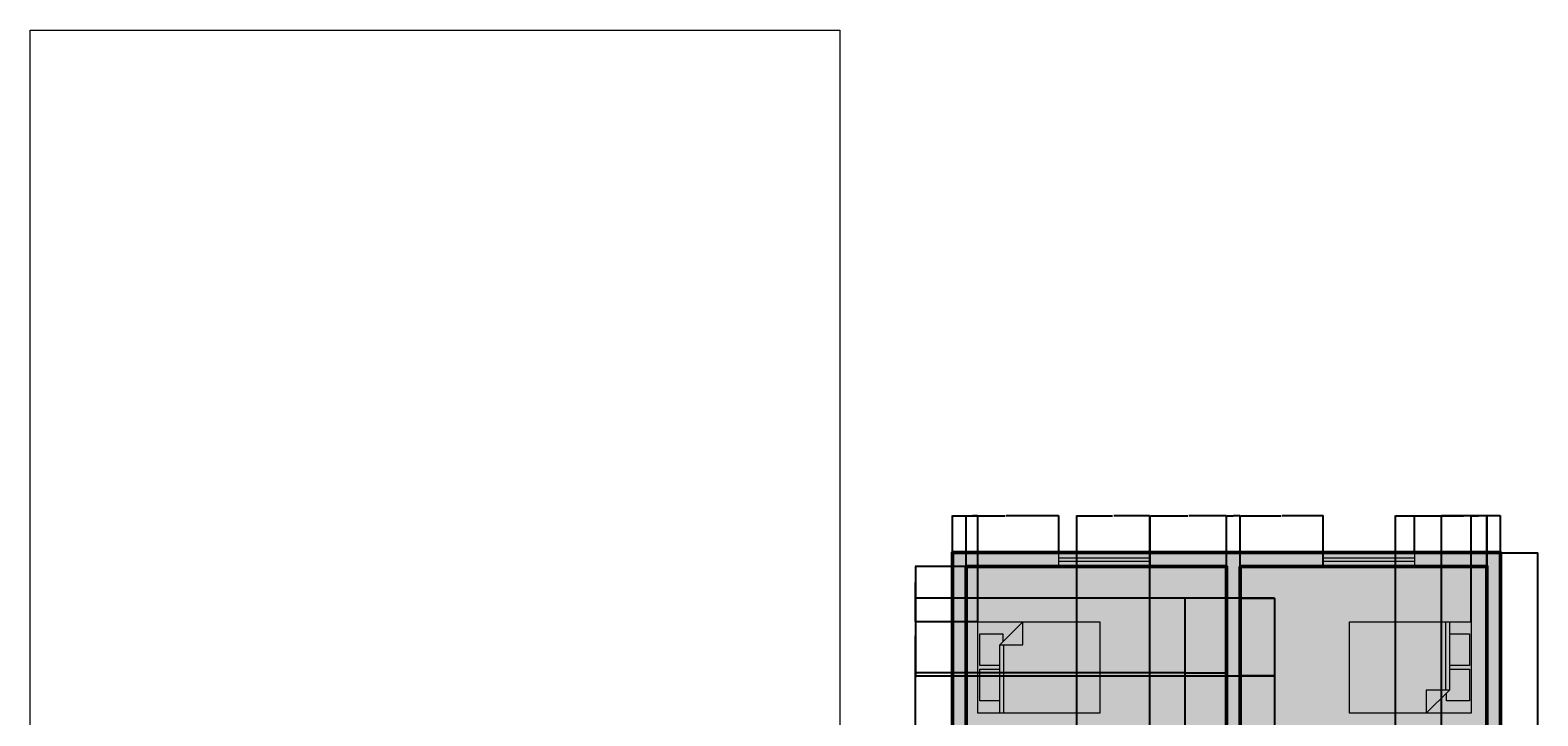
# Model space of a CAD drawing. Units: inches. Extents: x -494 to 1275, y 12 to 1194.
# Tile 4 of 8: x -494 to 496, y 743 to 1194. Entities that reach past the tile are written whole.
import ezdxf

# ---------------------------------------------------------------- set-up
doc = ezdxf.new("R2010")
doc.units = ezdxf.units.IN
doc.header["$MEASUREMENT"] = 0
for name, color, linetype, lineweight in [('A-ANNO-DIMS', 2, 'Continuous', 18), ('A-FLOR-CASE', 7, 'Continuous', 25), ('A-FURN', 8, 'Continuous', 18), ('A-GLAZ', 4, 'Continuous', 18), ('A-GLAZ-FRAM-PATT', 7, 'Continuous', 13), ('A-GLAZ-GLAS-PATT', 4, 'Continuous', 13), ('A-REF-IMAG', 8, 'Continuous', 13), ('A-WALL', 7, 'Continuous', 50)]:
    doc.layers.add(name, color=color, linetype=linetype, lineweight=lineweight)
for name, color, linetype, lineweight, true_color in [('A-FLOR-CASE-PATT', 31, 'Continuous', 13, 0xfecc66), ('A-FLOR-PATT', 51, 'Continuous', 13, 0xf8f6b0), ('A-FURN-PATT', 254, 'Continuous', 13, 0xfeeab9), ('A-WALL-PATT', 251, 'Continuous', 13, 0x636466)]:
    doc.layers.add(name, color=color, linetype=linetype, lineweight=lineweight, true_color=true_color)
doc.styles.get("Standard").update_dxf_attribs({"font": 'arial.ttf'})
doc.dimstyles.get("Standard").update_dxf_attribs({"dimtxt": 0.18, "dimasz": 0.18, "dimexe": 0.18, "dimexo": 0.0625, "dimgap": 0.09, "dimtad": 0, "dimtih": 1, "dimtoh": 1, "dimdec": 4, "dimzin": 0, "dimdsep": 46, "dimlunit": 4, "dimtxsty": 'Standard', "dimcen": 0.09, "dimadec": 0, "dimazin": 0, "dimtfac": 1, "dimtdec": 4, "dimtofl": 0, "dimtmove": 0, "dimatfit": 3, "dimfxl": 1, "dimtolj": 1, "dimtzin": 0, "dimarcsym": 0})
picture_1 = doc.add_image_def('image1.jpeg', size_in_pixel=(720, 1600))

# ---------------------------------------------------------------- blocks, each defined once
blk = doc.blocks.new('Bed - Queen')
for p, q in [((0, -80.00003), (0, 0)), ((0, 0), (59.99999, 0)), ((59.99999, 0), (59.99999, -80.00003)), ((7.99999, -1.2), (28.79998, -1.2)), ((7.99999, -14.4), (7.99999, -1.2)), ((28.79998, -1.2), (28.79998, -14.4)), ((31.19999, -1.2), (51.99999, -1.2)), ((31.19999, -14.4), (31.19999, -1.2)), ((51.99999, -1.2), (51.99999, -16.4)), ((0, -14.4), (44.8, -14.4)), ((44.8, -16.8), (0, -16.8)), ((59.99999, -29.6), (44.8, -14.4)), ((44.8, -14.4), (44.8, -29.6)), ((51.99999, -16.4), (46.79936, -16.4)), ((44.8, -29.6), (59.99999, -29.6)), ((59.99999, -80.00003), (0, -80.00003))]:
    blk.add_line(p, q)
blk = doc.blocks.new('WINDOW-60IN')
for p, q in [((3.5, 60), (3.5, 0)), ((5.5, 60), (5.5, 0))]:
    blk.add_line(p, q)
blk.add_lwpolyline([(9, 0), (0, 0), (0, 60), (9, 60)], close=True)
blk = doc.blocks.new('*D43')
at = {"layer": 'A-ANNO-DIMS', "color": 0, "lineweight": -2, "transparency": 16777216}
for p, q in [((471.79, 850.53), (496.16, 850.53)), ((495.98, 850.35), (495.98, 610.72)), ((495.98, 370.71), (495.98, 610.35)), ((471.79, 370.53), (496.16, 370.53))]:
    blk.add_line(p, q, dxfattribs=at)
at = {"layer": 'A-ANNO-DIMS', "color": 0, "transparency": 16777216}
for points in [[(495.95, 850.35), (496.01, 850.35), (495.98, 850.53)], [(495.95, 370.71), (496.01, 370.71), (495.98, 370.53)]]:
    blk.add_solid(points, dxfattribs=at)
at = {"layer": 'Defpoints', "color": 0, "transparency": 16777216}
for p in [(471.73, 850.53), (495.98, 850.53), (471.73, 370.53)]:
    blk.add_point(p, dxfattribs=at)
at = {"layer": 'A-ANNO-DIMS', "color": 0, "transparency": 16777216, "insert": (495.98, 610.53), "char_height": 0.18, "attachment_point": 5}
blk.add_mtext('\\A1;480', dxfattribs=at)
blk = doc.blocks.new('*D45')
at = {"layer": 'A-ANNO-DIMS', "color": 0, "lineweight": -2, "transparency": 16777216}
for p, q in [((120.67, 841.53), (87.3, 841.53)), ((87.48, 841.35), (87.48, 769.72)), ((87.48, 697.71), (87.48, 769.35)), ((120.67, 697.53), (87.3, 697.53))]:
    blk.add_line(p, q, dxfattribs=at)
at = {"layer": 'A-ANNO-DIMS', "color": 0, "transparency": 16777216}
for points in [[(87.45, 841.35), (87.51, 841.35), (87.48, 841.53)], [(87.45, 697.71), (87.51, 697.71), (87.48, 697.53)]]:
    blk.add_solid(points, dxfattribs=at)
at = {"layer": 'Defpoints', "color": 0, "transparency": 16777216}
for p in [(120.73, 841.53), (87.48, 697.53), (120.73, 697.53)]:
    blk.add_point(p, dxfattribs=at)
at = {"layer": 'A-ANNO-DIMS', "color": 0, "transparency": 16777216, "insert": (87.48, 769.53), "char_height": 0.18, "attachment_point": 5}
blk.add_mtext('\\A1;144', dxfattribs=at)
blk = doc.blocks.new('*D47')
at = {"layer": 'A-ANNO-DIMS', "color": 0, "lineweight": -2, "transparency": 16777216}
for p, q in [((111.73, 850.6), (111.73, 874.96)), ((111.91, 874.78), (146.31, 874.78)), ((181.46, 874.78), (147.06, 874.78)), ((181.64, 850.6), (181.64, 874.96))]:
    blk.add_line(p, q, dxfattribs=at)
at = {"layer": 'A-ANNO-DIMS', "color": 0, "transparency": 16777216}
for points in [[(111.91, 874.81), (111.91, 874.75), (111.73, 874.78)], [(181.46, 874.81), (181.46, 874.75), (181.64, 874.78)]]:
    blk.add_solid(points, dxfattribs=at)
at = {"layer": 'Defpoints', "color": 0, "transparency": 16777216}
for p in [(181.64, 874.78), (111.73, 850.53), (181.64, 850.53)]:
    blk.add_point(p, dxfattribs=at)
at = {"layer": 'A-ANNO-DIMS', "color": 0, "transparency": 16777216, "insert": (146.69, 874.78), "char_height": 0.18, "attachment_point": 5}
blk.add_mtext('\\A1;69.91', dxfattribs=at)
blk = doc.blocks.new('*D48')
at = {"layer": 'A-ANNO-DIMS', "color": 0, "lineweight": -2, "transparency": 16777216}
for p, q in [((241.64, 841.6), (241.64, 874.96)), ((241.82, 874.78), (266.29, 874.78)), ((291.55, 874.78), (267.08, 874.78)), ((291.73, 841.6), (291.73, 874.96))]:
    blk.add_line(p, q, dxfattribs=at)
at = {"layer": 'A-ANNO-DIMS', "color": 0, "transparency": 16777216}
for points in [[(241.82, 874.81), (241.82, 874.75), (241.64, 874.78)], [(291.55, 874.81), (291.55, 874.75), (291.73, 874.78)]]:
    blk.add_solid(points, dxfattribs=at)
at = {"layer": 'Defpoints', "color": 0, "transparency": 16777216}
for p in [(291.73, 874.78), (241.64, 841.53), (291.73, 841.53)]:
    blk.add_point(p, dxfattribs=at)
at = {"layer": 'A-ANNO-DIMS', "color": 0, "transparency": 16777216, "insert": (266.69, 874.78), "char_height": 0.18, "attachment_point": 5}
blk.add_mtext('\\A1;50.09', dxfattribs=at)
blk = doc.blocks.new('*D49')
at = {"layer": 'A-ANNO-DIMS', "color": 0, "lineweight": -2, "transparency": 16777216}
for p, q in [((300.73, 841.6), (300.73, 874.96)), ((300.91, 874.78), (327.62, 874.78)), ((355.11, 874.78), (328.4, 874.78)), ((355.29, 841.6), (355.29, 874.96))]:
    blk.add_line(p, q, dxfattribs=at)
at = {"layer": 'A-ANNO-DIMS', "color": 0, "transparency": 16777216}
for points in [[(300.91, 874.81), (300.91, 874.75), (300.73, 874.78)], [(355.11, 874.81), (355.11, 874.75), (355.29, 874.78)]]:
    blk.add_solid(points, dxfattribs=at)
at = {"layer": 'Defpoints', "color": 0, "transparency": 16777216}
for p in [(355.29, 874.78), (300.73, 841.53), (355.29, 841.53)]:
    blk.add_point(p, dxfattribs=at)
at = {"layer": 'A-ANNO-DIMS', "color": 0, "transparency": 16777216, "insert": (328.01, 874.78), "char_height": 0.18, "attachment_point": 5}
blk.add_mtext('\\A1;54.56', dxfattribs=at)
blk = doc.blocks.new('*D50')
at = {"layer": 'A-ANNO-DIMS', "color": 0, "lineweight": -2, "transparency": 16777216}
for p, q in [((415.29, 850.6), (415.29, 874.96)), ((415.47, 874.78), (443.12, 874.78)), ((471.55, 874.78), (443.9, 874.78)), ((471.73, 850.6), (471.73, 874.96))]:
    blk.add_line(p, q, dxfattribs=at)
at = {"layer": 'A-ANNO-DIMS', "color": 0, "transparency": 16777216}
for points in [[(415.47, 874.81), (415.47, 874.75), (415.29, 874.78)], [(471.55, 874.81), (471.55, 874.75), (471.73, 874.78)]]:
    blk.add_solid(points, dxfattribs=at)
at = {"layer": 'Defpoints', "color": 0, "transparency": 16777216}
for p in [(471.73, 874.78), (415.29, 850.53), (471.73, 850.53)]:
    blk.add_point(p, dxfattribs=at)
at = {"layer": 'A-ANNO-DIMS', "color": 0, "transparency": 16777216, "insert": (443.51, 874.78), "char_height": 0.18, "attachment_point": 5}
blk.add_mtext('\\A1;56.44', dxfattribs=at)
blk = doc.blocks.new('*D52')
at = {"layer": 'A-ANNO-DIMS', "color": 0, "lineweight": -2, "transparency": 16777216}
for p, q in [((193.38, 451.6), (193.38, 874.96)), ((193.56, 874.78), (216.96, 874.78)), ((241.16, 874.78), (217.76, 874.78)), ((241.34, 451.6), (241.34, 874.96))]:
    blk.add_line(p, q, dxfattribs=at)
at = {"layer": 'A-ANNO-DIMS', "color": 0, "transparency": 16777216}
for points in [[(193.56, 874.81), (193.56, 874.75), (193.38, 874.78)], [(241.16, 874.81), (241.16, 874.75), (241.34, 874.78)]]:
    blk.add_solid(points, dxfattribs=at)
at = {"layer": 'Defpoints', "color": 0, "transparency": 16777216}
for p in [(241.34, 874.78), (193.38, 451.53), (241.34, 451.53)]:
    blk.add_point(p, dxfattribs=at)
at = {"layer": 'A-ANNO-DIMS', "color": 0, "transparency": 16777216, "insert": (217.36, 874.78), "char_height": 0.18, "attachment_point": 5}
blk.add_mtext('\\A1;47.96', dxfattribs=at)
blk = doc.blocks.new('*D56')
at = {"layer": 'A-ANNO-DIMS', "color": 0, "lineweight": -2, "transparency": 16777216}
for p, q in [((402.73, 688.6), (402.73, 874.96)), ((402.91, 874.78), (432.51, 874.78)), ((462.55, 874.78), (432.95, 874.78)), ((462.73, 688.6), (462.73, 874.96))]:
    blk.add_line(p, q, dxfattribs=at)
at = {"layer": 'A-ANNO-DIMS', "color": 0, "transparency": 16777216}
for points in [[(402.91, 874.81), (402.91, 874.75), (402.73, 874.78)], [(462.55, 874.81), (462.55, 874.75), (462.73, 874.78)]]:
    blk.add_solid(points, dxfattribs=at)
at = {"layer": 'Defpoints', "color": 0, "transparency": 16777216}
for p in [(462.73, 874.78), (402.73, 688.53), (462.73, 688.53)]:
    blk.add_point(p, dxfattribs=at)
at = {"layer": 'A-ANNO-DIMS', "color": 0, "transparency": 16777216, "insert": (432.73, 874.78), "char_height": 0.18, "attachment_point": 5}
blk.add_mtext('\\A1;60', dxfattribs=at)
blk = doc.blocks.new('*D62')
at = {"layer": 'A-ANNO-DIMS', "color": 0, "lineweight": -2, "transparency": 16777216}
for p, q in [((291.73, 841.6), (291.73, 874.96)), ((291.91, 874.78), (296.08, 874.78)), ((300.55, 874.78), (296.38, 874.78)), ((300.73, 841.6), (300.73, 874.96))]:
    blk.add_line(p, q, dxfattribs=at)
at = {"layer": 'A-ANNO-DIMS', "color": 0, "transparency": 16777216}
for points in [[(291.91, 874.81), (291.91, 874.75), (291.73, 874.78)], [(300.55, 874.81), (300.55, 874.75), (300.73, 874.78)]]:
    blk.add_solid(points, dxfattribs=at)
at = {"layer": 'Defpoints', "color": 0, "transparency": 16777216}
for p in [(300.73, 874.78), (291.73, 841.53), (300.73, 841.53)]:
    blk.add_point(p, dxfattribs=at)
at = {"layer": 'A-ANNO-DIMS', "color": 0, "transparency": 16777216, "insert": (296.23, 874.78), "char_height": 0.18, "attachment_point": 5}
blk.add_mtext('\\A1;9', dxfattribs=at)
blk = doc.blocks.new('*D64')
at = {"layer": 'A-ANNO-DIMS', "color": 0, "lineweight": -2, "transparency": 16777216}
for p, q in [((432.84, 595.6), (432.84, 874.96)), ((433.02, 874.78), (447.43, 874.78)), ((462.76, 874.78), (448.35, 874.78)), ((462.94, 595.6), (462.94, 874.96))]:
    blk.add_line(p, q, dxfattribs=at)
at = {"layer": 'A-ANNO-DIMS', "color": 0, "transparency": 16777216}
for points in [[(433.02, 874.81), (433.02, 874.75), (432.84, 874.78)], [(462.76, 874.81), (462.76, 874.75), (462.94, 874.78)]]:
    blk.add_solid(points, dxfattribs=at)
at = {"layer": 'Defpoints', "color": 0, "transparency": 16777216}
for p in [(462.94, 874.78), (432.84, 595.53), (462.94, 595.53)]:
    blk.add_point(p, dxfattribs=at)
at = {"layer": 'A-ANNO-DIMS', "color": 0, "transparency": 16777216, "insert": (447.89, 874.78), "char_height": 0.18, "attachment_point": 5}
blk.add_mtext('\\A1;30.104', dxfattribs=at)
blk = doc.blocks.new('*D78')
at = {"layer": 'A-ANNO-DIMS', "color": 0, "lineweight": -2, "transparency": 16777216}
for p, q in [((120.67, 841.53), (87.3, 841.53)), ((87.48, 841.35), (87.48, 823.51)), ((87.48, 805.31), (87.48, 823.15)), ((128.44, 805.13), (87.3, 805.13))]:
    blk.add_line(p, q, dxfattribs=at)
at = {"layer": 'A-ANNO-DIMS', "color": 0, "transparency": 16777216}
for points in [[(87.45, 841.35), (87.51, 841.35), (87.48, 841.53)], [(87.45, 805.31), (87.51, 805.31), (87.48, 805.13)]]:
    blk.add_solid(points, dxfattribs=at)
at = {"layer": 'Defpoints', "color": 0, "transparency": 16777216}
for p in [(120.73, 841.53), (87.48, 805.13), (128.5, 805.13)]:
    blk.add_point(p, dxfattribs=at)
at = {"layer": 'A-ANNO-DIMS', "color": 0, "transparency": 16777216, "insert": (87.48, 823.33), "char_height": 0.18, "attachment_point": 5}
blk.add_mtext('\\A1;36.41', dxfattribs=at)
blk = doc.blocks.new('*D79')
at = {"layer": 'A-ANNO-DIMS', "color": 0, "lineweight": -2, "transparency": 16777216}
for p, q in [((120.73, 841.6), (120.73, 874.96)), ((120.91, 874.78), (124.22, 874.78)), ((128.32, 874.78), (125.01, 874.78)), ((128.5, 805.19), (128.5, 874.96))]:
    blk.add_line(p, q, dxfattribs=at)
at = {"layer": 'A-ANNO-DIMS', "color": 0, "transparency": 16777216}
for points in [[(120.91, 874.81), (120.91, 874.75), (120.73, 874.78)], [(128.32, 874.81), (128.32, 874.75), (128.5, 874.78)]]:
    blk.add_solid(points, dxfattribs=at)
at = {"layer": 'Defpoints', "color": 0, "transparency": 16777216}
for p in [(128.5, 874.78), (120.73, 841.53), (128.5, 805.13)]:
    blk.add_point(p, dxfattribs=at)
at = {"layer": 'A-ANNO-DIMS', "color": 0, "transparency": 16777216, "insert": (124.61, 874.78), "char_height": 0.18, "attachment_point": 5}
blk.add_mtext('\\A1;7.765', dxfattribs=at)
blk = doc.blocks.new('*D80')
at = {"layer": 'A-ANNO-DIMS', "color": 0, "lineweight": -2, "transparency": 16777216}
for p, q in [((452.5, 805.19), (452.5, 874.96)), ((452.68, 874.78), (457.16, 874.78)), ((462.55, 874.78), (458.07, 874.78)), ((462.73, 841.6), (462.73, 874.96))]:
    blk.add_line(p, q, dxfattribs=at)
at = {"layer": 'A-ANNO-DIMS', "color": 0, "transparency": 16777216}
for points in [[(452.68, 874.81), (452.68, 874.75), (452.5, 874.78)], [(462.55, 874.81), (462.55, 874.75), (462.73, 874.78)]]:
    blk.add_solid(points, dxfattribs=at)
at = {"layer": 'Defpoints', "color": 0, "transparency": 16777216}
for p in [(462.73, 874.78), (462.73, 841.53), (452.5, 805.13)]:
    blk.add_point(p, dxfattribs=at)
at = {"layer": 'A-ANNO-DIMS', "color": 0, "transparency": 16777216, "insert": (457.61, 874.78), "char_height": 0.18, "attachment_point": 5}
blk.add_mtext('\\A1;10.234', dxfattribs=at)
blk = doc.blocks.new('*D81')
at = {"layer": 'A-ANNO-DIMS', "color": 0, "lineweight": -2, "transparency": 16777216}
for p, q in [((291.67, 841.53), (87.3, 841.53)), ((87.48, 841.35), (87.48, 831.22)), ((87.48, 820.72), (87.48, 830.86)), ((291.67, 820.54), (87.3, 820.54))]:
    blk.add_line(p, q, dxfattribs=at)
at = {"layer": 'A-ANNO-DIMS', "color": 0, "transparency": 16777216}
for points in [[(87.45, 841.35), (87.51, 841.35), (87.48, 841.53)], [(87.45, 820.72), (87.51, 820.72), (87.48, 820.54)]]:
    blk.add_solid(points, dxfattribs=at)
at = {"layer": 'Defpoints', "color": 0, "transparency": 16777216}
for p in [(291.73, 841.53), (87.48, 820.54), (291.73, 820.54)]:
    blk.add_point(p, dxfattribs=at)
at = {"layer": 'A-ANNO-DIMS', "color": 0, "transparency": 16777216, "insert": (87.48, 831.04), "char_height": 0.18, "attachment_point": 5}
blk.add_mtext('\\A1;20.99', dxfattribs=at)
blk = doc.blocks.new('*D82')
at = {"layer": 'A-ANNO-DIMS', "color": 0, "lineweight": -2, "transparency": 16777216}
for p, q in [((264.34, 820.48), (264.34, 346.1)), ((291.73, 820.48), (291.73, 346.1)), ((264.52, 346.28), (277.57, 346.28)), ((291.55, 346.28), (278.5, 346.28))]:
    blk.add_line(p, q, dxfattribs=at)
at = {"layer": 'A-ANNO-DIMS', "color": 0, "transparency": 16777216}
for points in [[(264.52, 346.31), (264.52, 346.25), (264.34, 346.28)], [(291.55, 346.31), (291.55, 346.25), (291.73, 346.28)]]:
    blk.add_solid(points, dxfattribs=at)
at = {"layer": 'Defpoints', "color": 0, "transparency": 16777216}
for p in [(264.34, 820.54), (291.73, 820.54), (291.73, 346.28)]:
    blk.add_point(p, dxfattribs=at)
at = {"layer": 'A-ANNO-DIMS', "color": 0, "transparency": 16777216, "insert": (278.04, 346.28), "char_height": 0.18, "attachment_point": 5}
blk.add_mtext('\\A1;27.394', dxfattribs=at)
blk = doc.blocks.new('*D83')
at = {"layer": 'A-ANNO-DIMS', "color": 0, "lineweight": -2, "transparency": 16777216}
for p, q in [((300.73, 820.48), (300.73, 346.1)), ((323.29, 820.48), (323.29, 346.1)), ((300.91, 346.28), (311.55, 346.28)), ((323.11, 346.28), (312.48, 346.28))]:
    blk.add_line(p, q, dxfattribs=at)
at = {"layer": 'A-ANNO-DIMS', "color": 0, "transparency": 16777216}
for points in [[(300.91, 346.31), (300.91, 346.25), (300.73, 346.28)], [(323.11, 346.31), (323.11, 346.25), (323.29, 346.28)]]:
    blk.add_solid(points, dxfattribs=at)
at = {"layer": 'Defpoints', "color": 0, "transparency": 16777216}
for p in [(300.73, 820.54), (323.29, 820.54), (323.29, 346.28)]:
    blk.add_point(p, dxfattribs=at)
at = {"layer": 'A-ANNO-DIMS', "color": 0, "transparency": 16777216, "insert": (312.01, 346.28), "char_height": 0.18, "attachment_point": 5}
blk.add_mtext('\\A1;22.557', dxfattribs=at)
blk = doc.blocks.new('*D84')
at = {"layer": 'A-ANNO-DIMS', "color": 0, "lineweight": -2, "transparency": 16777216}
for p, q in [((264.28, 820.54), (87.3, 820.54)), ((87.48, 820.36), (87.48, 796.22)), ((87.48, 771.72), (87.48, 795.86)), ((264.28, 771.54), (87.3, 771.54))]:
    blk.add_line(p, q, dxfattribs=at)
at = {"layer": 'A-ANNO-DIMS', "color": 0, "transparency": 16777216}
for points in [[(87.45, 820.36), (87.51, 820.36), (87.48, 820.54)], [(87.45, 771.72), (87.51, 771.72), (87.48, 771.54)]]:
    blk.add_solid(points, dxfattribs=at)
at = {"layer": 'Defpoints', "color": 0, "transparency": 16777216}
for p in [(87.48, 820.54), (264.34, 820.54), (264.34, 771.54)]:
    blk.add_point(p, dxfattribs=at)
at = {"layer": 'A-ANNO-DIMS', "color": 0, "transparency": 16777216, "insert": (87.48, 796.04), "char_height": 0.18, "attachment_point": 5}
blk.add_mtext('\\A1;49', dxfattribs=at)
blk = doc.blocks.new('*D85')
at = {"layer": 'A-ANNO-DIMS', "color": 0, "lineweight": -2, "transparency": 16777216}
for p, q in [((323.23, 820.54), (87.3, 820.54)), ((87.48, 820.36), (87.48, 795.22)), ((87.48, 769.71), (87.48, 794.86)), ((323.23, 769.53), (87.3, 769.53))]:
    blk.add_line(p, q, dxfattribs=at)
at = {"layer": 'A-ANNO-DIMS', "color": 0, "transparency": 16777216}
for points in [[(87.45, 820.36), (87.51, 820.36), (87.48, 820.54)], [(87.45, 769.71), (87.51, 769.71), (87.48, 769.53)]]:
    blk.add_solid(points, dxfattribs=at)
at = {"layer": 'Defpoints', "color": 0, "transparency": 16777216}
for p in [(87.48, 820.54), (323.29, 820.54), (323.29, 769.53)]:
    blk.add_point(p, dxfattribs=at)
at = {"layer": 'A-ANNO-DIMS', "color": 0, "transparency": 16777216, "insert": (87.48, 795.04), "char_height": 0.18, "attachment_point": 5}
blk.add_mtext('\\A1;51.01', dxfattribs=at)

msp = doc.modelspace()

# ---------------------------------------------------------------- hatches: boundary and pattern name
at = {"layer": 'A-FLOR-CASE-PATT'}
h = msp.add_hatch(dxfattribs=at)
h.set_pattern_fill('ANGLE', color=256)
h.set_pattern_definition([(0, (-187.50956, -172.72298), (0, 0.275), [0.2, -0.075]), (90, (-187.50956, -172.72298), (-0.275, 0), [0.2, -0.075])])
h.paths.add_polyline_path([(291.7322, 820.5433), (264.338, 820.5433), (264.338, 771.5415), (291.7322, 771.5415)])
h.paths.add_polyline_path([(323.2889, 820.5433), (300.7322, 820.5433), (300.7322, 769.5349), (323.2889, 769.5349)])
at = {"layer": 'A-FLOR-PATT'}
h = msp.add_hatch(color=256, dxfattribs=at)
h.dxf.hatch_style = 1
h.paths.add_polyline_path([(333.7322, 595.5349), (393.7322, 595.5349), (393.7322, 617.1185), (393.7322, 653.1185), (393.7322, 688.5349), (348.3096, 688.5349), (348.3096, 697.5349), (462.7322, 697.5349), (462.7322, 841.5349), (300.7322, 841.5349), (300.7322, 820.5433), (323.2889, 820.5433), (323.2889, 769.5349), (300.7322, 769.5349), (300.7322, 697.5349), (312.3096, 697.5349), (312.3096, 688.5349), (276.4565, 688.5349), (276.4565, 697.5349), (291.7322, 697.5349), (291.7322, 771.5415), (264.338, 771.5415), (264.338, 820.5433), (291.7322, 820.5433), (291.7322, 841.5349), (120.7322, 841.5349), (120.7322, 697.5349), (240.4565, 697.5349), (240.4565, 688.5349), (120.7322, 688.5349), (120.7322, 451.5349), (241.3385, 451.5349), (241.3385, 442.5349), (277.3385, 442.5349), (277.3385, 451.5349), (333.7322, 451.5349), (333.7322, 473.4986), (333.7322, 509.4986)])
h.paths.add_polyline_path([(372.4977, 745.1275), (372.4977, 805.1275), (452.4977, 805.1275), (452.4977, 745.1275)], flags=16)
h.paths.add_polyline_path([(208.4976, 745.1275), (128.4976, 745.1275), (128.4976, 805.1275), (208.4976, 805.1275)], flags=16)
h.paths.add_polyline_path([(422.8977, 745.1275), (422.8977, 760.3275), (438.0977, 760.3275), (438.0977, 797.1275), (451.2977, 797.1275), (451.2977, 776.3275), (438.0977, 776.3275), (438.0977, 773.9275), (451.2977, 773.9275), (451.2977, 753.1275), (436.0977, 753.1275), (436.0977, 758.3275)], flags=16)
h.paths.add_polyline_path([(142.8976, 789.9275), (142.8976, 753.1275), (129.6976, 753.1275), (129.6976, 773.9275), (142.8976, 773.9275), (142.8976, 776.3275), (129.6976, 776.3275), (129.6976, 797.1275), (144.8976, 797.1275), (144.8976, 791.9275), (158.0976, 805.1275), (158.0976, 789.9275)], flags=0)
at = {"layer": 'A-FURN-PATT'}
h = msp.add_hatch(color=256, dxfattribs=at)
h.dxf.hatch_style = 1
h.paths.add_polyline_path([(158.0976, 805.1275), (128.4976, 805.1275), (128.4976, 745.1275), (142.8976, 745.1275), (142.8976, 753.1275), (129.6976, 753.1275), (129.6976, 773.9275), (142.8976, 773.9275), (142.8976, 776.3275), (129.6976, 776.3275), (129.6976, 797.1275), (144.8976, 797.1275), (144.8976, 791.9275)])
h = msp.add_hatch(color=256, dxfattribs=at)
h.dxf.hatch_style = 1
h.paths.add_polyline_path([(158.0976, 805.1275), (142.8976, 789.9275), (158.0976, 789.9275)])
h.paths.add_polyline_path([(145.2976, 789.9275), (142.8976, 789.9275), (142.8976, 745.1275), (145.2976, 745.1275)])
h = msp.add_hatch(color=256, dxfattribs=at)
h.dxf.hatch_style = 1
h.paths.add_polyline_path([(208.4976, 805.1275), (158.0976, 805.1275), (158.0976, 789.9275), (145.2976, 789.9275), (145.2976, 745.1275), (208.4976, 745.1275)])
h.paths.add_polyline_path([(435.6977, 805.1275), (372.4977, 805.1275), (372.4977, 745.1275), (422.8977, 745.1275), (422.8977, 760.3275), (435.6977, 760.3275)])
h = msp.add_hatch(color=256, dxfattribs=at)
h.dxf.hatch_style = 1
h.paths.add_polyline_path([(452.4977, 805.1275), (438.0977, 805.1275), (438.0977, 797.1275), (451.2977, 797.1275), (451.2977, 776.3275), (438.0977, 776.3275), (438.0977, 773.9275), (451.2977, 773.9275), (451.2977, 753.1275), (436.0977, 753.1275), (436.0977, 758.3275), (422.8977, 745.1275), (452.4977, 745.1275)])
h = msp.add_hatch(color=256, dxfattribs=at)
h.dxf.hatch_style = 1
h.paths.add_polyline_path([(438.0977, 805.1275), (435.6977, 805.1275), (435.6977, 760.3275), (438.0977, 760.3275)])
h = msp.add_hatch(color=256, dxfattribs=at)
h.dxf.hatch_style = 1
h.paths.add_polyline_path([(129.6976, 776.3275), (142.8976, 776.3275), (142.8976, 789.9275), (144.8976, 791.9275), (144.8976, 797.1275), (129.6976, 797.1275)])
h.paths.add_polyline_path([(129.6976, 753.1275), (142.8976, 753.1275), (142.8976, 773.9275), (129.6976, 773.9275)])
h = msp.add_hatch(color=256, dxfattribs=at)
h.dxf.hatch_style = 1
h.paths.add_polyline_path([(129.6976, 776.3275), (142.8976, 776.3275), (142.8976, 789.9275), (144.8976, 791.9275), (144.8976, 797.1275), (129.6976, 797.1275)])
h.paths.add_polyline_path([(129.6976, 753.1275), (142.8976, 753.1275), (142.8976, 773.9275), (129.6976, 773.9275)])
h = msp.add_hatch(color=256, dxfattribs=at)
h.dxf.hatch_style = 1
h.paths.add_polyline_path([(451.2977, 773.9275), (438.0977, 773.9275), (438.0977, 760.3275), (436.0977, 758.3275), (436.0977, 753.1275), (451.2977, 753.1275)])
h.paths.add_polyline_path([(451.2977, 797.1275), (438.0977, 797.1275), (438.0977, 776.3275), (451.2977, 776.3275)])
h = msp.add_hatch(color=256, dxfattribs=at)
h.dxf.hatch_style = 1
h.paths.add_polyline_path([(438.0977, 760.3275), (422.8977, 760.3275), (422.8977, 745.1275)])
at = {"layer": 'A-GLAZ-FRAM-PATT'}
h = msp.add_hatch(color=256, dxfattribs=at)
h.dxf.hatch_style = 1
h.paths.add_polyline_path([(241.6425, 850.5349), (181.6425, 850.5349), (181.6425, 847.0349), (241.6425, 847.0349)])
h.paths.add_polyline_path([(241.6425, 845.0349), (181.6425, 845.0349), (181.6425, 841.5349), (241.6425, 841.5349)])
h = msp.add_hatch(color=256, dxfattribs=at)
h.dxf.hatch_style = 1
h.paths.add_polyline_path([(415.2879, 850.5349), (355.2879, 850.5349), (355.2879, 847.0349), (415.2879, 847.0349)])
h.paths.add_polyline_path([(415.2879, 845.0349), (355.2879, 845.0349), (355.2879, 841.5349), (415.2879, 841.5349)])
at = {"layer": 'A-GLAZ-GLAS-PATT'}
h = msp.add_hatch(color=256, dxfattribs=at)
h.dxf.hatch_style = 1
h.paths.add_polyline_path([(241.6425, 847.0349), (181.6425, 847.0349), (181.6425, 845.0349), (241.6425, 845.0349)])
h = msp.add_hatch(color=256, dxfattribs=at)
h.dxf.hatch_style = 1
h.paths.add_polyline_path([(415.2879, 847.0349), (355.2879, 847.0349), (355.2879, 845.0349), (415.2879, 845.0349)])
at = {"layer": 'A-WALL-PATT'}
h = msp.add_hatch(color=256, dxfattribs=at)
h.dxf.hatch_style = 1
h.paths.add_polyline_path([(120.7322, 841.5349), (291.7322, 841.5349), (291.7322, 697.5349), (276.4565, 697.5349), (276.4565, 688.5349), (312.3096, 688.5349), (312.3096, 697.5349), (300.7322, 697.5349), (300.7322, 841.5349), (462.7322, 841.5349), (462.7322, 697.5349), (348.3096, 697.5349), (348.3096, 688.5349), (393.7322, 688.5349), (393.7322, 653.1185), (402.7322, 653.1185), (402.7322, 688.5349), (462.7322, 688.5349), (462.7322, 604.5349), (402.7322, 604.5349), (402.7322, 617.1185), (393.7322, 617.1185), (393.7322, 595.5349), (333.7322, 595.5349), (333.7322, 509.4986), (342.7322, 509.4986), (342.7322, 586.5349), (393.7322, 586.5349), (402.7322, 586.5349), (402.7322, 595.5349), (462.9409, 595.5349), (462.7406, 379.5349), (342.7322, 379.5349), (342.7322, 442.5349), (342.7322, 473.4986), (333.7322, 473.4986), (333.7322, 451.5349), (277.3385, 451.5349), (277.3385, 442.5349), (333.7322, 442.5349), (333.7322, 370.5349), (471.7322, 370.5349), (471.7322, 850.5349), (111.7322, 850.5349), (111.7322, 442.5349), (241.3385, 442.5349), (241.3385, 451.5349), (120.7322, 451.5349), (120.7322, 688.5349), (240.4565, 688.5349), (240.4565, 697.5349), (120.7322, 697.5349)])

# ---------------------------------------------------------------- linework, layer by layer
at = {"layer": 'A-FLOR-CASE'}
for p, q in [((291.7322, 820.5433), (264.338, 820.5433)), ((264.338, 820.5433), (264.338, 771.5415)), ((300.7322, 820.5433), (323.2889, 820.5433)), ((323.2889, 820.5433), (323.2889, 769.5349)), ((264.338, 771.5415), (291.7322, 771.5415)), ((323.2889, 769.5349), (300.7322, 769.5349))]:
    msp.add_line(p, q, dxfattribs=at)
at = {"layer": 'A-WALL'}
for points in [[(333.7322, 442.5349), (333.7322, 370.5349), (471.7322, 370.5349), (471.7322, 850.5349), (111.7322, 850.5349), (111.7322, 442.5349), (241.3385, 442.5349), (241.3385, 451.5349), (120.7322, 451.5349), (120.7322, 688.5349), (240.4565, 688.5349), (240.4565, 697.5349), (120.7322, 697.5349), (120.7322, 841.5349), (291.7322, 841.5349), (291.7322, 697.5349), (276.4565, 697.5349), (276.4565, 688.5349), (312.3096, 688.5349), (312.3096, 697.5349), (300.7322, 697.5349), (300.7322, 841.5349)], [(462.9409, 595.5349), (402.7322, 595.5349), (402.7322, 586.5349), (393.7322, 586.5349), (342.7322, 586.5349), (342.7322, 509.4986), (333.7322, 509.4986), (333.7322, 595.5349), (393.7322, 595.5349), (393.7322, 617.1185), (402.7322, 617.1185), (402.7322, 604.5349), (462.7322, 604.5349), (462.7322, 688.5349), (402.7322, 688.5349), (402.7322, 653.1185), (393.7322, 653.1185), (393.7322, 688.5349), (348.3096, 688.5349), (348.3096, 697.5349), (462.7322, 697.5349), (462.7322, 841.5349), (300.7322, 841.5349)]]:
    msp.add_lwpolyline(points, dxfattribs=at)

# ---------------------------------------------------------------- block references
at = {"layer": 'A-FURN'}
for p, rotation in [((128.4976, 745.1275), 89.99999999999999), ((128.4976, 745.1275), 90), ((452.4977, 805.1275), 270)]:
    msp.add_blockref('Bed - Queen', p, dxfattribs=dict(at, rotation=rotation))
at = {"layer": 'A-GLAZ', "rotation": 89.99999999999976}
for p in [(241.642, 841.5346), (415.2874, 841.5346)]:
    msp.add_blockref('WINDOW-60IN', p, dxfattribs=at)

# ---------------------------------------------------------------- dimensions: what is measured, and where the dimension line sits
at = {"layer": 'A-ANNO-DIMS'}
for base, p1, p2, override, picture, middle in [((181.6425, 874.7849), (111.7322, 850.5349), (181.6425, 850.5349), {"dimdec": 2, "dimlfac": 1, "dimrnd": 0, "dimzin": 0, "dimdsep": 46, "dimlunit": 2}, '*D47', (146.6873, 874.7849)), ((128.4976, 874.7849), (120.7322, 841.5349), (128.4976, 805.1275), {"dimdec": 3, "dimlfac": 1, "dimrnd": 0, "dimzin": 0, "dimdsep": 46, "dimlunit": 2}, '*D79', (124.6149, 874.7849)), ((241.3385, 874.7849), (193.3783, 451.5349), (241.3385, 451.5349), {"dimdec": 2, "dimlfac": 1, "dimrnd": 0, "dimzin": 0, "dimdsep": 46, "dimlunit": 2}, '*D52', (217.3584, 874.7849)), ((291.7322, 874.7849), (241.6425, 841.5349), (291.7322, 841.5349), {"dimdec": 2, "dimlfac": 1, "dimrnd": 0, "dimzin": 0, "dimdsep": 46, "dimlunit": 2}, '*D48', (266.6873, 874.7849)), ((300.7322, 874.7849), (291.7322, 841.5349), (300.7322, 841.5349), {"dimdec": 0, "dimlfac": 1, "dimrnd": 0, "dimzin": 0, "dimdsep": 46, "dimlunit": 2}, '*D62', (296.2322, 874.7849)), ((355.2879, 874.7849), (300.7322, 841.5349), (355.2879, 841.5349), {"dimdec": 2, "dimlfac": 1, "dimrnd": 0, "dimzin": 0, "dimdsep": 46, "dimlunit": 2}, '*D49', (328.01, 874.7849)), ((462.7322, 874.7849), (402.7322, 688.5349), (462.7322, 688.5349), {"dimdec": 0, "dimlfac": 1, "dimrnd": 0, "dimzin": 0, "dimdsep": 46, "dimlunit": 2}, '*D56', (432.7322, 874.7849)), ((471.7322, 874.7849), (415.2879, 850.5349), (471.7322, 850.5349), {"dimdec": 2, "dimlfac": 1, "dimrnd": 0, "dimzin": 0, "dimdsep": 46, "dimlunit": 2}, '*D50', (443.51, 874.7849)), ((462.9409, 874.7849), (432.8366, 595.5349), (462.9409, 595.5349), {"dimdec": 3, "dimlfac": 1, "dimrnd": 0, "dimzin": 0, "dimdsep": 46, "dimlunit": 2}, '*D64', (447.8888, 874.7849)), ((462.73221, 874.78491), (452.49775, 805.1275), (462.73221, 841.53491), {"dimdec": 3, "dimlfac": 1, "dimrnd": 0, "dimzin": 0, "dimdsep": 46, "dimlunit": 2}, '*D80', (457.61498, 874.78491)), ((291.7322, 346.2849), (264.338, 820.5433), (291.7322, 820.5433), {"dimdec": 3, "dimlfac": 1, "dimrnd": 0, "dimzin": 0, "dimdsep": 46, "dimlunit": 2}, '*D82', (278.0351, 346.2849)), ((323.2889, 346.2849), (300.7322, 820.5433), (323.2889, 820.5433), {"dimdec": 3, "dimlfac": 1, "dimrnd": 0, "dimzin": 0, "dimdsep": 46, "dimlunit": 2}, '*D83', (312.0106, 346.2849))]:
    dim = msp.add_linear_dim(base=base, p1=p1, p2=p2, dimstyle='Standard', override=override, dxfattribs=at)
    dim.commit()
    dim.dimension.update_dxf_attribs({"geometry": picture, "text_midpoint": middle})
for base, p1, p2, override, picture, middle in [((87.4822, 805.1275), (120.7322, 841.5349), (128.4976, 805.1275), {"dimdec": 2, "dimlfac": 1, "dimrnd": 0, "dimzin": 0, "dimdsep": 46, "dimlunit": 2}, '*D78', (87.4822, 823.3312)), ((87.4822, 820.5433), (291.7322, 841.5349), (291.7322, 820.5433), {"dimdec": 2, "dimlfac": 1, "dimrnd": 0, "dimzin": 0, "dimdsep": 46, "dimlunit": 2}, '*D81', (87.4822, 831.0391)), ((87.4822, 697.5349), (120.7322, 841.5349), (120.7322, 697.5349), {"dimdec": 0, "dimlfac": 1, "dimrnd": 0, "dimzin": 0, "dimdsep": 46, "dimlunit": 2}, '*D45', (87.4822, 769.5349)), ((495.9822, 850.5349), (471.7322, 370.5349), (471.7322, 850.5349), {"dimdec": 0, "dimlfac": 1, "dimrnd": 0, "dimzin": 0, "dimdsep": 46, "dimlunit": 2}, '*D43', (495.9822, 610.5349)), ((87.4822, 820.5433), (323.2889, 769.5349), (323.2889, 820.5433), {"dimdec": 2, "dimlfac": 1, "dimrnd": 0, "dimzin": 0, "dimdsep": 46, "dimlunit": 2}, '*D85', (87.4822, 795.0391)), ((87.4822, 820.5433), (264.338, 771.5415), (264.338, 820.5433), {"dimdec": 0, "dimlfac": 1, "dimrnd": 0, "dimzin": 0, "dimdsep": 46, "dimlunit": 2}, '*D84', (87.4822, 796.0424))]:
    dim = msp.add_linear_dim(base=base, p1=p1, p2=p2, angle=90, dimstyle='Standard', override=override, dxfattribs=at)
    dim.commit()
    dim.dimension.update_dxf_attribs({"geometry": picture, "text_midpoint": middle})

# ---------------------------------------------------------------- pictures from other files: only their frames are drawn
at = {"layer": 'A-REF-IMAG'}
image = msp.add_image(picture_1, insert=(-493.8358, 12.0215), size_in_units=(531.7593, 1181.6872), dxfattribs=at)
image.dxf.flags = 7

doc.saveas('drawing.dxf')
